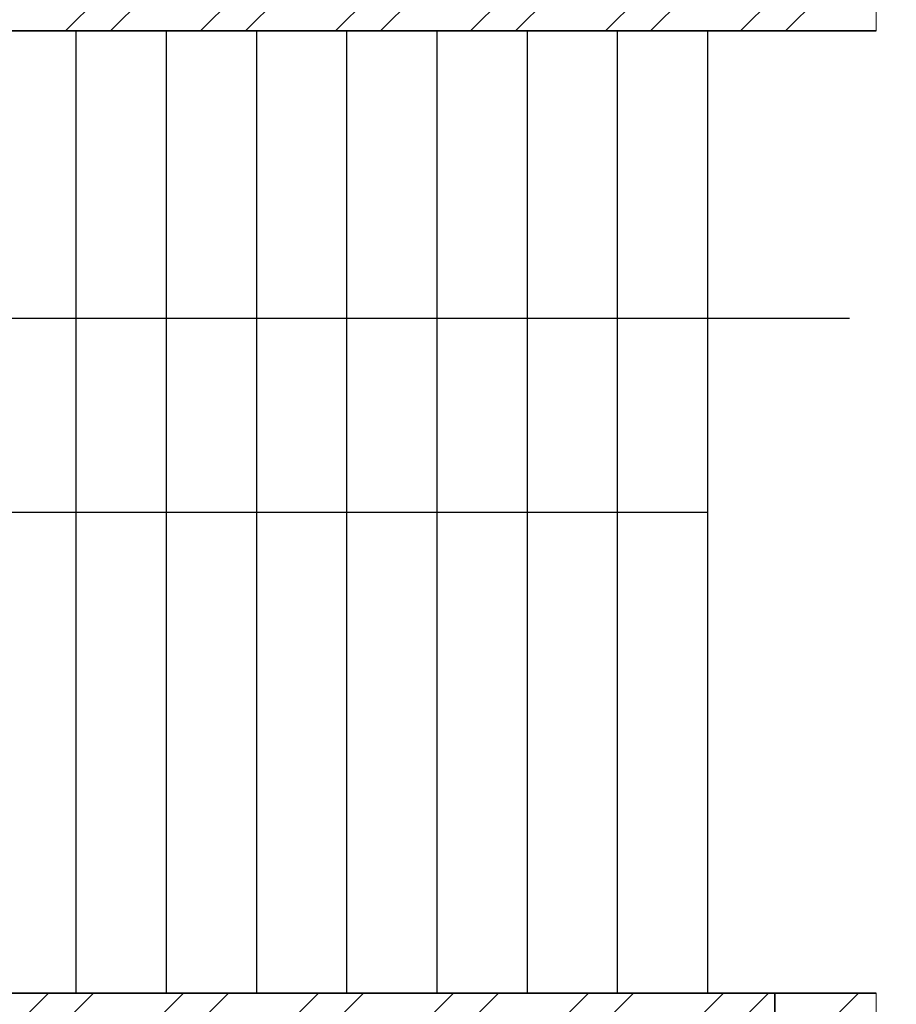
# Model space of a CAD drawing. Units: inches. Extents: x 1962 to 2771, y 1245 to 2660.
# Tile 36 of 114: x 2159 to 2247, y 1932 to 2030. Entities that reach past the tile are written whole.
import ezdxf

# ---------------------------------------------------------------- set-up
doc = ezdxf.new("R2010")
doc.units = ezdxf.units.IN
for name, color, linetype, lineweight in [('A-DOOR', 3, 'Continuous', 18), ('A-FLOR-STRS', 7, 'Continuous', 25), ('A-WALL', 7, 'Continuous', 35), ('A-WALL-PATT', 252, 'Continuous', 13)]:
    doc.layers.add(name, color=color, linetype=linetype, lineweight=lineweight)

msp = doc.modelspace()

# ---------------------------------------------------------------- hatches: boundary and pattern name
at = {"layer": 'A-WALL-PATT'}
h = msp.add_hatch(dxfattribs=at)
h.set_pattern_fill('ANSI32', color=256)
h.paths.add_polyline_path([(2090.8074, 2467.3437), (2141.6481, 2467.3437), (2141.6481, 2469.5937), (2141.6481, 2471.8437), (2086.3074, 2471.8437), (2086.3074, 2422.5333), (2090.8074, 2422.5333)])
h.paths.add_polyline_path([(2282.7664, 2471.8437), (2204.8982, 2471.8437), (2204.8982, 2467.3437), (2234.8074, 2467.3437), (2234.8074, 2311.3437), (2228.7492, 2311.3437), (2228.7492, 2306.8437), (2234.8074, 2306.8437), (2331.9227, 2306.8437), (2331.9227, 2309.0937), (2331.9227, 2311.3437), (2239.3074, 2311.3437), (2239.3074, 2467.3437), (2282.7664, 2467.3437), (2282.7664, 2469.5937)])
h.paths.add_polyline_path([(2471.4531, 2519.8437), (2552.011, 2519.8437), (2564.3996, 2519.8437), (2564.3996, 2511.1389), (2568.8996, 2511.1389), (2568.8996, 2524.3437), (2466.9531, 2524.3437), (2466.9531, 2471.8437), (2450.0749, 2471.8437), (2446.4672, 2471.8437), (2446.4672, 2467.3437), (2450.0749, 2467.3437), (2475.9988, 2467.3437), (2475.9988, 2469.5937), (2475.9988, 2471.8437), (2471.4531, 2471.8437)])
h.paths.add_polyline_path([(2575.2231, 2469.5937), (2575.2231, 2471.8437), (2568.8996, 2471.8437), (2568.8996, 2487.1389), (2564.3996, 2487.1389), (2564.3996, 2471.8437), (2556.511, 2471.8437), (2499.2904, 2471.8437), (2499.2904, 2467.3437), (2507.8074, 2467.3437), (2507.8074, 2311.3437), (2414.863, 2311.3437), (2414.863, 2306.8437), (2512.3074, 2306.8437), (2517.0114, 2306.8437), (2517.0114, 2309.0937), (2517.0114, 2311.3437), (2512.3074, 2311.3437), (2512.3074, 2467.3437), (2575.2231, 2467.3437)])
h.paths.add_polyline_path([(2660.8074, 2471.8437), (2600.9602, 2471.8437), (2600.9602, 2467.3437), (2656.3074, 2467.3437), (2656.3074, 2432.5704), (2660.8074, 2432.5704)])
h.paths.add_polyline_path([(2660.8074, 2372.5704), (2656.3074, 2372.5704), (2656.3074, 2311.3437), (2600.276, 2311.3437), (2600.276, 2309.0937), (2600.276, 2306.8437), (2656.3074, 2306.8437), (2656.3074, 2296.2593), (2660.8074, 2296.2593)])
h.paths.add_polyline_path([(2572.3074, 2306.8437), (2577.1385, 2306.8437), (2577.1385, 2311.3437), (2551.082, 2311.3437), (2551.082, 2306.8437), (2567.8074, 2306.8437), (2567.8074, 2258.8437), (2540.0574, 2258.8437), (2540.0574, 2256.5937), (2540.0574, 2254.3437), (2567.8074, 2254.3437), (2656.3074, 2254.3437), (2656.3074, 2236.9085), (2660.8074, 2236.9085), (2660.8074, 2272.2593), (2656.3074, 2272.2593), (2656.3074, 2258.8437), (2572.3074, 2258.8437)])
h.paths.add_polyline_path([(2512.3074, 2254.3437), (2518.8716, 2254.3437), (2518.8716, 2256.5937), (2518.8716, 2258.8437), (2507.8074, 2258.8437), (2507.8074, 2177.8437), (2567.8074, 2177.8437), (2567.8074, 2172.9628), (2572.3074, 2172.9628), (2572.3074, 2177.8437), (2656.3074, 2177.8437), (2656.3074, 2166.4846), (2660.8074, 2166.4846), (2660.8074, 2200.9085), (2656.3074, 2200.9085), (2656.3074, 2182.3437), (2512.3074, 2182.3437)])
h.paths.add_polyline_path([(2656.3074, 2129.8437), (2572.3074, 2129.8437), (2572.3074, 2150.3044), (2570.0574, 2150.3044), (2567.8074, 2150.3044), (2567.8074, 2129.8437), (2507.8074, 2129.8437), (2507.8074, 2116.3027), (2510.0574, 2116.3027), (2512.3074, 2116.3027), (2512.3074, 2125.3437), (2567.8074, 2125.3437), (2572.3074, 2125.3437), (2656.3074, 2125.3437)])
h.paths.add_polyline_path([(2090.8074, 2362.5333), (2086.3074, 2362.5333), (2086.3074, 2298.6242), (2090.8074, 2298.6242), (2090.8074, 2306.8437), (2174.8074, 2306.8437), (2174.8074, 2286.4178), (2179.3074, 2286.4178), (2179.3074, 2306.8437), (2192.8641, 2306.8437), (2192.8641, 2309.0937), (2192.8641, 2311.3437), (2090.8074, 2311.3437)])
h.paths.add_polyline_path([(2209.156, 2258.8437), (2179.3074, 2258.8437), (2179.3074, 2263.2236), (2177.0574, 2263.2236), (2174.8074, 2263.2236), (2174.8074, 2258.8437), (2090.8074, 2258.8437), (2090.8074, 2274.6242), (2086.3074, 2274.6242), (2086.3074, 2238.2967), (2088.5574, 2238.2967), (2090.8074, 2238.2967), (2090.8074, 2254.3437), (2209.156, 2254.3437)])
h.paths.add_polyline_path([(2090.8074, 2177.8437), (2234.8074, 2177.8437), (2234.8074, 2173.1428), (2239.3074, 2173.1428), (2239.3074, 2258.8437), (2230.8442, 2258.8437), (2230.8442, 2256.5937), (2230.8442, 2254.3437), (2234.8074, 2254.3437), (2234.8074, 2182.3437), (2090.8074, 2182.3437), (2090.8074, 2202.2967), (2086.3074, 2202.2967), (2086.3074, 2140.0389), (2090.8074, 2140.0389)])
h.paths.add_polyline_path([(2090.8074, 2080.0389), (2086.3074, 2080.0389), (2086.3074, 2033.8437), (2090.8074, 2033.8437)], flags=17)
h.paths.add_polyline_path([(2244.9405, 2033.8437), (2239.3074, 2033.8437), (2239.3074, 2142.0665), (2237.2592, 2142.0665), (2234.8074, 2142.0665), (2234.8074, 2033.8437), (2090.8074, 2033.8437), (2076.5204, 2033.8437), (2072.0204, 2033.8437), (2072.0204, 2000.4493), (2076.5204, 2000.4493), (2076.5204, 2029.3437), (2090.8074, 2029.3437), (2244.9405, 2029.3437), (2244.9405, 2031.5937)])
h.paths.add_polyline_path([(2234.8074, 1933.3437), (2076.5204, 1933.3437), (2076.5204, 1952.4493), (2074.2704, 1952.4493), (2072.0204, 1952.4493), (2072.0204, 1933.3437), (2072.0204, 1928.8437), (2234.8074, 1928.8437)])
h.paths.add_polyline_path([(2090.8074, 1928.8437), (2086.3074, 1928.8437), (2086.3074, 1906.5013), (2090.8074, 1906.5013)])
h.paths.add_polyline_path([(2090.8074, 1846.5013), (2086.3074, 1846.5013), (2086.3074, 1769.9917), (2088.5574, 1769.9917), (2090.8074, 1769.9917), (2090.8074, 1780.3437), (2234.8074, 1780.3437), (2234.8074, 1708.3437), (2230.3764, 1708.3437), (2230.3764, 1703.8437), (2239.3074, 1703.8437), (2239.3074, 1792.6669), (2237.0574, 1792.6669), (2234.8074, 1792.6669), (2234.8074, 1784.8437), (2090.8074, 1784.8437)])
h.paths.add_polyline_path([(2239.3074, 1928.8437), (2244.9405, 1928.8437), (2244.9405, 1931.0937), (2244.9405, 1933.3437), (2234.8074, 1933.3437), (2234.8074, 1928.8437), (2234.8074, 1825.5949), (2239.3074, 1825.5949)])
h.paths.add_polyline_path([(2148.0425, 1649.0937), (2148.0425, 1651.3437), (2090.8074, 1651.3437), (2090.8074, 1646.8437), (2148.0425, 1646.8437)], flags=0)
h.paths.add_polyline_path([(2207.5601, 1708.3437), (2090.8074, 1708.3437), (2090.8074, 1703.8437), (2174.8074, 1703.8437), (2174.8074, 1651.3437), (2170.4457, 1651.3437), (2170.4457, 1646.8437), (2195.9924, 1646.8437), (2195.9924, 1649.0937), (2195.9924, 1651.3437), (2179.3074, 1651.3437), (2179.3074, 1703.8437), (2207.5601, 1703.8437), (2207.5601, 1706.0937)])
h.paths.add_polyline_path([(2090.8074, 1733.9917), (2086.3074, 1733.9917), (2086.3074, 1696.1032), (2088.5574, 1696.1032), (2090.8074, 1696.1032)])
h.paths.add_polyline_path([(2090.8074, 1672.1032), (2086.3074, 1672.1032), (2086.3074, 1600.3335), (2090.8074, 1600.3335)])
h.paths.add_polyline_path([(2090.8074, 1540.3335), (2086.3074, 1540.3335), (2086.3074, 1486.3437), (2139.6766, 1486.3437), (2139.6766, 1490.8437), (2090.8074, 1490.8437)])
h.paths.add_polyline_path([(2302.3876, 1490.8437), (2239.3074, 1490.8437), (2239.3074, 1646.8437), (2335.9994, 1646.8437), (2335.9994, 1651.3437), (2229.884, 1651.3437), (2229.884, 1646.8437), (2234.8074, 1646.8437), (2234.8074, 1490.8437), (2202.7103, 1490.8437), (2202.7103, 1488.5937), (2202.7103, 1486.3437), (2275.0699, 1486.3437), (2275.0699, 1475.772), (2279.5699, 1475.772), (2279.5699, 1486.3437), (2302.3876, 1486.3437)])
h.paths.add_polyline_path([(2279.5699, 1451.772), (2275.0699, 1451.772), (2275.0699, 1438.3437), (2174.8074, 1438.3437), (2174.8074, 1486.3437), (2179.7922, 1486.3437), (2179.7922, 1490.8437), (2163.3585, 1490.8437), (2163.3585, 1488.5937), (2163.3585, 1486.3437), (2170.3074, 1486.3437), (2170.3074, 1433.8437), (2279.5699, 1433.8437)])
h.paths.add_polyline_path([(2427.2363, 1490.8437), (2375.8074, 1490.8437), (2375.8074, 1646.8437), (2381.6401, 1646.8437), (2381.6401, 1651.3437), (2365.887, 1651.3437), (2365.887, 1649.0937), (2365.887, 1646.8437), (2371.3074, 1646.8437), (2371.3074, 1490.8437), (2327.5627, 1490.8437), (2327.5627, 1488.5937), (2327.5627, 1486.3437), (2371.3074, 1486.3437), (2371.3074, 1433.8437), (2375.8074, 1433.8437), (2375.8074, 1486.3437), (2427.2363, 1486.3437)])
h.paths.add_polyline_path([(2512.3074, 1646.8437), (2519.4351, 1646.8437), (2519.4351, 1649.0937), (2519.4351, 1651.3437), (2507.8074, 1651.3437), (2416.0063, 1651.3437), (2416.0063, 1649.0937), (2416.0063, 1646.8437), (2507.8074, 1646.8437), (2507.8074, 1490.8437), (2497.0532, 1490.8437), (2497.0532, 1488.5937), (2497.0532, 1486.3437), (2574.9344, 1486.3437), (2574.9344, 1476.0181), (2579.4344, 1476.0181), (2579.4344, 1486.3437), (2584.4872, 1486.3437), (2584.3074, 1490.8437), (2512.3074, 1490.8437)])
h.paths.add_polyline_path([(2470.5091, 1486.3437), (2473.9767, 1486.3437), (2473.9767, 1490.8437), (2449.6605, 1490.8437), (2449.6605, 1488.5937), (2449.6605, 1486.3437), (2466.0091, 1486.3437), (2466.0091, 1433.8437), (2470.5091, 1433.8437), (2579.4344, 1433.8437), (2579.4344, 1452.0181), (2574.9344, 1452.0181), (2574.9344, 1438.3437), (2554.5091, 1438.3437), (2470.5091, 1438.3437)])
h.paths.add_polyline_path([(2656.3074, 1490.8437), (2611.86, 1490.8437), (2611.86, 1486.3437), (2656.3074, 1486.3437)])
h.paths.add_polyline_path([(2660.8074, 1532.7007), (2658.5574, 1532.7007), (2656.3074, 1532.7007), (2656.3074, 1486.3437), (2660.8074, 1486.3437)])
h.paths.add_polyline_path([(2660.8074, 1664.9663), (2656.3074, 1664.9663), (2656.3074, 1651.3437), (2602.2313, 1651.3437), (2602.2313, 1646.8437), (2656.3074, 1646.8437), (2656.3074, 1592.7007), (2660.8074, 1592.7007)])
h.paths.add_polyline_path([(2660.8074, 1724.5221), (2656.3074, 1724.5221), (2656.3074, 1703.8437), (2542.4725, 1703.8437), (2542.4725, 1699.3437), (2567.8074, 1699.3437), (2567.8074, 1651.3437), (2552.7766, 1651.3437), (2552.7766, 1649.0937), (2552.7766, 1646.8437), (2577.2878, 1646.8437), (2577.2878, 1649.0937), (2577.2878, 1651.3437), (2572.3074, 1651.3437), (2572.3074, 1699.3437), (2656.3074, 1699.3437), (2656.3074, 1688.9663), (2660.8074, 1688.9663)])
h.paths.add_polyline_path([(2660.8074, 1880.6524), (2656.3074, 1880.6524), (2656.3074, 1832.8437), (2512.3074, 1832.8437), (2512.3074, 1837.8959), (2507.8074, 1837.8959), (2507.8074, 1828.3437), (2567.8074, 1828.3437), (2567.8074, 1804.3437), (2572.3074, 1804.3437), (2572.3074, 1828.3437), (2656.3074, 1828.3437), (2656.3074, 1818.6778), (2660.8074, 1818.6778)])
h.paths.add_polyline_path([(2660.8074, 1794.6778), (2656.3074, 1794.6778), (2656.3074, 1780.3437), (2572.3074, 1780.3437), (2572.3074, 1783.0303), (2570.0574, 1783.0303), (2567.8074, 1783.0303), (2567.8074, 1780.3437), (2507.8074, 1780.3437), (2507.8074, 1699.3437), (2517.8858, 1699.3437), (2517.8858, 1701.5937), (2517.8858, 1703.8437), (2512.3074, 1703.8437), (2512.3074, 1775.8437), (2656.3074, 1775.8437), (2656.3074, 1760.5221), (2660.8074, 1760.5221)])
h.paths.add_polyline_path([(2660.8074, 1981.3437), (2660.8074, 2020.2808), (2658.5574, 2020.2808), (2656.3074, 2020.2808), (2656.3074, 1981.3437), (2512.3074, 1981.3437), (2512.3074, 2086.6996), (2507.8074, 2086.6996), (2507.8074, 1981.3437), (2375.8074, 1981.3437), (2375.8074, 1986.8505), (2373.5574, 1986.8505), (2371.3074, 1986.8505), (2371.3074, 1973.2607), (2375.8074, 1973.2607), (2375.8074, 1976.8437), (2507.8074, 1976.8437), (2507.8074, 1865.4281), (2510.0574, 1865.4281), (2512.3074, 1865.4281), (2512.3074, 1976.8437), (2660.8074, 1976.8437)])
h.paths.add_polyline_path([(2375.8074, 1940.297), (2373.5574, 1940.297), (2371.3074, 1940.297), (2371.3074, 1933.3437), (2278.4434, 1933.3437), (2278.4434, 1928.8437), (2371.3074, 1928.8437), (2371.3074, 1651.3437), (2375.8074, 1651.3437)])
h.paths.add_polyline_path([(2660.8074, 1976.8437), (2656.3074, 1976.8437), (2656.3074, 1940.6524), (2660.8074, 1940.6524)], flags=17)
h.paths.add_polyline_path([(2660.8074, 2142.4846), (2656.3074, 2142.4846), (2656.3074, 2080.2808), (2660.8074, 2080.2808)])
h.paths.add_polyline_path([(2381.4189, 2311.3437), (2375.8074, 2311.3437), (2375.8074, 2467.3437), (2424.7242, 2467.3437), (2424.7242, 2469.5937), (2424.7242, 2471.8437), (2375.8074, 2471.8437), (2375.8074, 2524.3437), (2371.3074, 2524.3437), (2371.3074, 2471.8437), (2307.2097, 2471.8437), (2307.2097, 2467.3437), (2371.3074, 2467.3437), (2371.3074, 2311.3437), (2366.8901, 2311.3437), (2366.8901, 2306.8437), (2371.3074, 2306.8437), (2371.3074, 2033.8437), (2279.6589, 2033.8437), (2279.6589, 2029.3437), (2371.3074, 2029.3437), (2371.3074, 2014.2598), (2375.8074, 2014.2598), (2375.8074, 2306.8437), (2381.4189, 2306.8437)])
h.paths.add_polyline_path([(2263.3074, 2524.3437), (2170.3074, 2524.3437), (2170.3074, 2519.8437), (2170.3074, 2471.8437), (2165.0312, 2471.8437), (2165.0312, 2467.3437), (2179.6721, 2467.3437), (2179.6721, 2469.5161), (2179.6721, 2471.8437), (2174.8074, 2471.8437), (2174.8074, 2519.8437), (2258.8074, 2519.8437), (2258.8074, 2511.6436), (2263.3074, 2511.6436)])
h.paths.add_polyline_path([(2245.0232, 1361.4123), (2492.9468, 1361.4123), (2492.9468, 1398.505), (2245.0232, 1398.505)], flags=9)
h.paths.add_polyline_path([(2388.1434, 2086.6936), (2425.0704, 2086.6936), (2425.0704, 2105.3509), (2388.1434, 2105.3509)], flags=9)
h.paths.add_polyline_path([(2404.922, 2242.6744), (2445.7337, 2242.6744), (2445.7337, 2261.3318), (2404.922, 2261.3318)], flags=9)
h.paths.add_polyline_path([(2269.4107, 2156.7935), (2306.3378, 2156.7935), (2306.3378, 2175.4508), (2269.4107, 2175.4508)], flags=9)
h.paths.add_polyline_path([(2269.3277, 2233.4343), (2306.2547, 2233.4343), (2306.2547, 2252.0917), (2269.3277, 2252.0917)], flags=9)
h.paths.add_polyline_path([(2431.6052, 2320.6922), (2470.4456, 2320.6922), (2470.4456, 2339.3495), (2431.6052, 2339.3495)], flags=25)
h.paths.add_polyline_path([(2249.6902, 2315.7608), (2288.5306, 2315.7608), (2288.5306, 2334.4182), (2249.6902, 2334.4182)], flags=25)
h.paths.add_polyline_path([(2096.9301, 2314.3181), (2135.7704, 2314.3181), (2135.7704, 2332.9755), (2096.9301, 2332.9755)], flags=25)
h.paths.add_polyline_path([(2134.3475, 2285.7089), (2161.4655, 2285.7089), (2161.4655, 2304.3662), (2134.3475, 2304.3662)], flags=9)
h.paths.add_polyline_path([(2126.5155, 2209.4076), (2159.9227, 2209.4076), (2159.9227, 2228.065), (2126.5155, 2228.065)], flags=25)
h.paths.add_polyline_path([(2110.5753, 2141.5299), (2149.4157, 2141.5299), (2149.4157, 2160.1872), (2110.5753, 2160.1872)], flags=25)
h.paths.add_polyline_path([(2249.8618, 1968.3317), (2286.3966, 1968.3317), (2286.3966, 1986.989), (2249.8618, 1986.989)], flags=9)
h.paths.add_polyline_path([(2395.9507, 1777.0051), (2436.7624, 1777.0051), (2436.7624, 1795.6625), (2395.9507, 1795.6625)], flags=9)
h.paths.add_polyline_path([(2398.5259, 1888.5651), (2435.0062, 1888.5651), (2435.0062, 1907.2224), (2398.5259, 1907.2224)], flags=25)
h.paths.add_polyline_path([(2259.3506, 1728.3559), (2296.2776, 1728.3559), (2296.2776, 1747.0132), (2259.3506, 1747.0132)], flags=9)
h.paths.add_polyline_path([(2271.3698, 1845.268), (2308.2968, 1845.268), (2308.2968, 1863.9253), (2271.3698, 1863.9253)], flags=9)
h.paths.add_polyline_path([(2120.9355, 1786.3027), (2159.7759, 1786.3027), (2159.7759, 1804.9601), (2120.9355, 1804.9601)], flags=25)
h.paths.add_polyline_path([(2121.3164, 1732.1043), (2154.7236, 1732.1043), (2154.7236, 1750.7616), (2121.3164, 1750.7616)], flags=25)
h.paths.add_polyline_path([(2118.3706, 1678.8997), (2147.5282, 1678.8997), (2147.5282, 1697.557), (2118.3706, 1697.557)], flags=25)
h.paths.add_polyline_path([(2385.9227, 1493.557), (2424.763, 1493.557), (2424.763, 1512.2143), (2385.9227, 1512.2143)], flags=25)
h.paths.add_polyline_path([(2248.7058, 1500.0256), (2287.5462, 1500.0256), (2287.5462, 1518.6829), (2248.7058, 1518.6829)], flags=25)
h.paths.add_polyline_path([(2104.1669, 1617.3771), (2143.0073, 1617.3771), (2143.0073, 1636.0344), (2104.1669, 1636.0344)], flags=9)
h.paths.add_polyline_path([(2096.0714, 1447.8824), (2137.3845, 1447.8824), (2137.3845, 1458.1859), (2096.0714, 1458.1859)], flags=9)
h.paths.add_polyline_path([(2180.6114, 1440.325), (2209.7689, 1440.325), (2209.7689, 1458.9823), (2180.6114, 1458.9823)], flags=25)
h.paths.add_polyline_path([(2316.1698, 1447.9637), (2357.4829, 1447.9637), (2357.4829, 1458.2673), (2316.1698, 1458.2673)], flags=9)
h.paths.add_polyline_path([(2397.6187, 1447.9637), (2438.9318, 1447.9637), (2438.9318, 1458.2673), (2397.6187, 1458.2673)], flags=9)
h.paths.add_polyline_path([(2473.0778, 1439.5953), (2502.2354, 1439.5953), (2502.2354, 1458.2527), (2473.0778, 1458.2527)], flags=25)
h.paths.add_polyline_path([(2589.7027, 1447.8819), (2631.0158, 1447.8819), (2631.0158, 1458.1855), (2589.7027, 1458.1855)], flags=9)
h.paths.add_polyline_path([(2522.4009, 1497.5285), (2561.2413, 1497.5285), (2561.2413, 1516.1859), (2522.4009, 1516.1859)], flags=25)
h.paths.add_polyline_path([(2579.6565, 1671.3482), (2608.8141, 1671.3482), (2608.8141, 1690.0056), (2579.6565, 1690.0056)], flags=25)
h.paths.add_polyline_path([(2544.7038, 1725.5064), (2578.1111, 1725.5064), (2578.1111, 1744.1637), (2544.7038, 1744.1637)], flags=25)
h.paths.add_polyline_path([(2578.1191, 1807.472), (2607.2766, 1807.472), (2607.2766, 1826.1293), (2578.1191, 1826.1293)], flags=25)
h.paths.add_polyline_path([(2595.0614, 1835.1839), (2633.9018, 1835.1839), (2633.9018, 1853.8413), (2595.0614, 1853.8413)], flags=25)
h.paths.add_polyline_path([(2567.0097, 2097.7035), (2605.8501, 2097.7035), (2605.8501, 2116.3609), (2567.0097, 2116.3609)], flags=9)
h.paths.add_polyline_path([(2586.644, 2134.6454), (2615.8015, 2134.6454), (2615.8015, 2153.3027), (2586.644, 2153.3027)], flags=9)
h.paths.add_polyline_path([(2544.6185, 2212.6783), (2578.0258, 2212.6783), (2578.0258, 2231.3356), (2544.6185, 2231.3356)], flags=25)
h.paths.add_polyline_path([(2577.0273, 2256.9023), (2606.1849, 2256.9023), (2606.1849, 2275.5597), (2577.0273, 2275.5597)], flags=24)
h.paths.add_polyline_path([(2605.2683, 2315.2821), (2644.1087, 2315.2821), (2644.1087, 2333.9395), (2605.2683, 2333.9395)], flags=25)
h.paths.add_polyline_path([(2583.1244, 2496.1815), (2624.4375, 2496.1815), (2624.4375, 2506.4851), (2583.1244, 2506.4851)], flags=9)
h.paths.add_polyline_path([(2474.761, 2497.0823), (2503.9185, 2497.0823), (2503.9185, 2515.7397), (2474.761, 2515.7397)], flags=25)
h.paths.add_polyline_path([(2387.5787, 2494.2563), (2428.902, 2494.2563), (2428.902, 2504.5598), (2387.5787, 2504.5598)], flags=9)
h.paths.add_polyline_path([(2300.1657, 2500.1564), (2341.4788, 2500.1564), (2341.4788, 2510.46), (2300.1657, 2510.46)], flags=25)
h.paths.add_polyline_path([(2176.8589, 2497.5843), (2206.0165, 2497.5843), (2206.0165, 2516.2416), (2176.8589, 2516.2416)], flags=25)
h.paths.add_polyline_path([(2097.4668, 2494.9762), (2138.7799, 2494.9762), (2138.7799, 2505.2798), (2097.4668, 2505.2798)], flags=9)

# ---------------------------------------------------------------- linework, layer by layer
at = {"layer": 'A-DOOR'}
for p, q in [((2244.9405, 2033.8437), (2244.9405, 2029.3437)), ((2244.9405, 2029.3437), (2244.9405, 2031.5937)), ((2244.9405, 1933.3437), (2244.9405, 1928.8437))]:
    msp.add_line(p, q, dxfattribs=at)
at = {"layer": 'A-FLOR-STRS'}
for p, q in [((2165.0955, 2029.3437), (2165.0955, 1933.3437)), ((2174.0955, 2029.3437), (2174.0955, 1933.3437)), ((2183.0955, 2029.3437), (2183.0955, 1933.3437)), ((2192.0955, 2029.3437), (2192.0955, 1933.3437)), ((2201.0955, 2029.3437), (2201.0955, 1933.3437)), ((2210.0955, 2029.3437), (2210.0955, 1933.3437)), ((2219.0955, 2029.3437), (2219.0955, 1933.3437)), ((2228.0955, 2029.3437), (2228.0955, 1933.3437)), ((2242.2648, 2000.646), (2096.9843, 2000.646)), ((2111.0955, 1981.3437), (2228.0955, 1981.3437))]:
    msp.add_line(p, q, dxfattribs=at)
at = {"layer": 'A-WALL'}
for p, q in [((2090.8074, 2029.3437), (2244.9405, 2029.3437)), ((2076.5204, 1933.3437), (2244.9405, 1933.3437)), ((2234.8074, 1933.3437), (2234.8074, 1824.0006))]:
    msp.add_line(p, q, dxfattribs=at)

doc.saveas('drawing.dxf')
